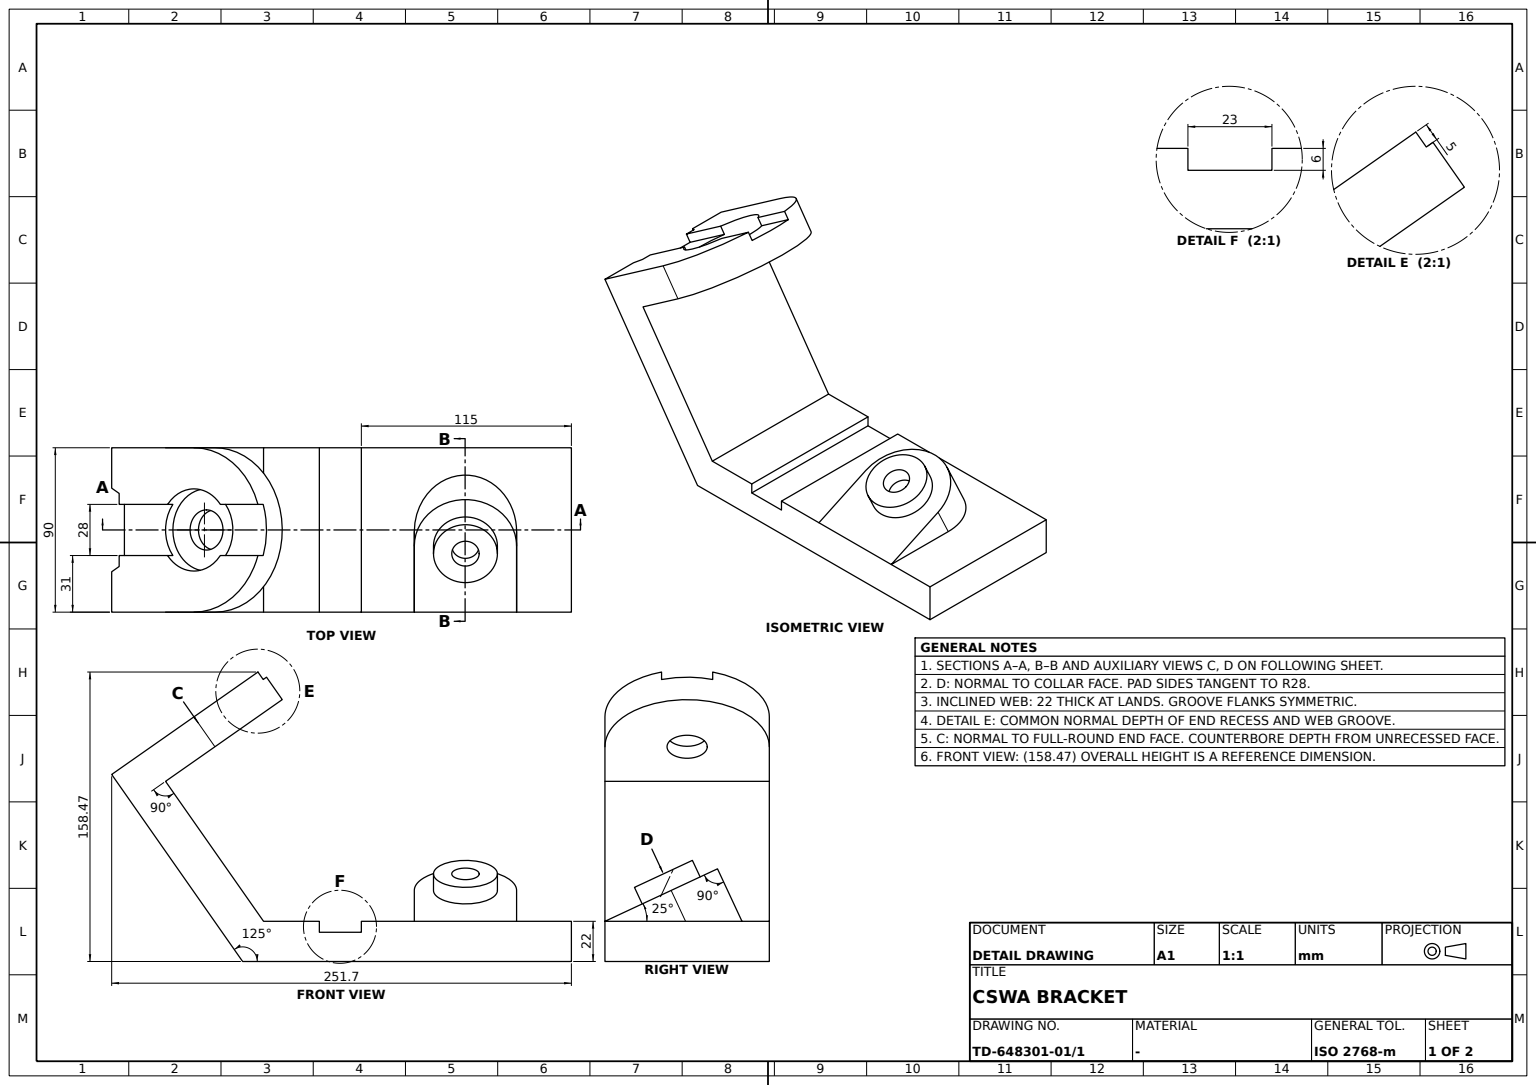
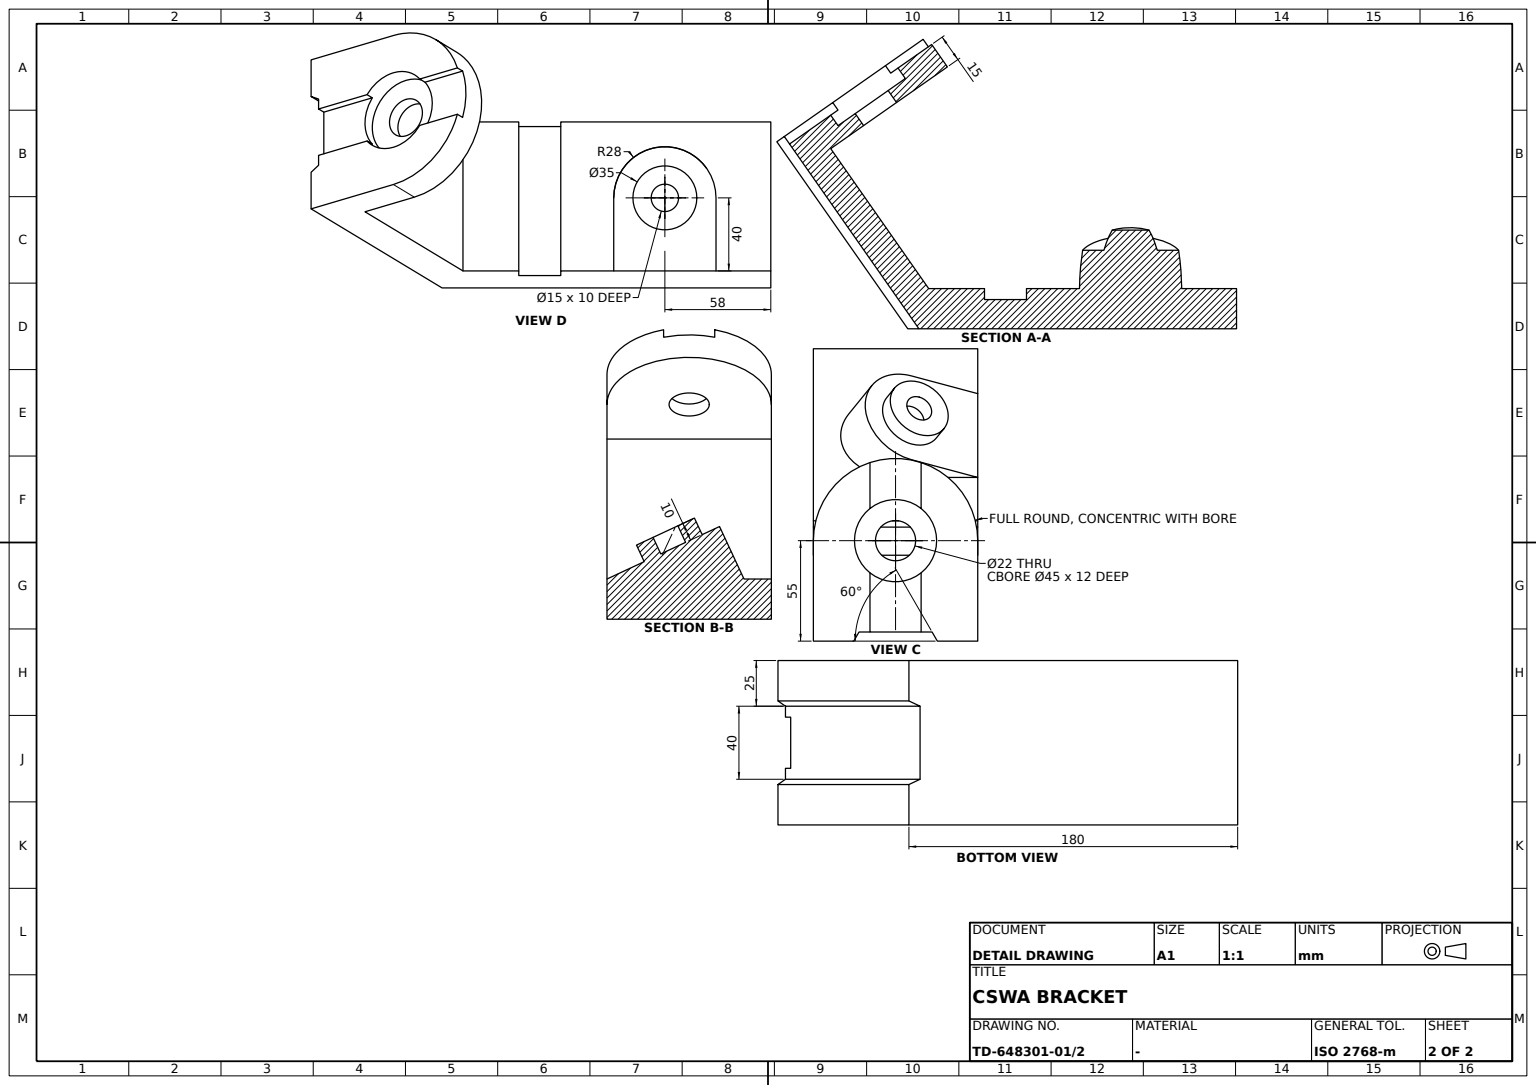
CATIA V5 part; units mm, degrees
ref_plane "Plane1" through (16.4638, 0, 35.3067) normal (-0.4226, 0, -0.9063) x (0, -1, 0)
sketch "Sketch1" plane through (0, 0, 0) normal (1, 0, 0) x (0, 1, 0)
  line L0 (0, 0) -> (180, 0)
  line L1 (180, 0) -> (180, 22)
  point P0 (180, 22)
  line L2 (0, 0) -> (-71.6971, 102.394)
  line L3 (-71.6971, 102.394) -> (-26.6437, 133.9407)
  line L4 (-26.6437, 133.9407) -> (-15.1722, 117.5577)
  point P1 (-15.1722, 117.5577)
  line L5 (-15.1722, 117.5577) -> (-42.2042, 98.6296)
  point P2 (-15.1722, 117.5577)
  point P3 (-42.2042, 98.6296)
  line L6 (-42.2042, 98.6296) -> (11.4525, 22)
  line L7 (11.4525, 22) -> (42, 22)
  point P4 (42, 22)
  line L8 (42, 22) -> (42, 16)
  line L9 (42, 16) -> (65, 16)
  line L10 (65, 16) -> (65, 22)
  point P5 (65, 22)
  line L11 (65, 22) -> (180, 22)
  dimension "length L0" = 180
  dimension "length L2" = 125
  dimension "angle L2 L0" = 55
  dimension "length L3" = 55
  dimension "length L4" = 20
  dimension "distance P3 L2" = 22
  dimension "distance P4 P0" = 138
  dimension "distance L7 L0" = 22
  dimension "length L8" = 6
  dimension "length L9" = 23
  constraint horizontal L0 x-axis
  constraint horizontal L7 x-axis
  constraint horizontal L9 x-axis
  constraint horizontal L11 x-axis
  constraint vertical L1 y-axis
  constraint vertical L8 y-axis
  constraint vertical L10 y-axis
  constraint perpendicularity L3 L2
  constraint parallelism L4 L2
  constraint parallelism L5 L3
  constraint parallelism L6 L2
  constraint coincidence P2 L4
  constraint coincidence P2 P1
  constraint coincidence P5 L7
extrude "Pad1" add sketch "Sketch1" along normal mid plane 90
sketch "Sketch2" plane through (16.4638, 0, 35.3067) normal (-0.4226, 0, -0.9063) x (0, -1, 0)
  line L0 (-150, -31.4862) -> (-150, 8.5138)
  point P0 (-150, -31.4862)
  line L1 (-180, -31.4862) -> (-65, -31.4862) construction
  line L2 (-180, 50.0815) -> (-180, -31.4862) construction
  line L3 (-94, 8.5138) -> (-94, -31.4862)
  arc A0 (-94, 8.5138) -> (-150, 8.5138) centre (-122, 8.5138) ccw
  line L4 (-94, -31.4862) -> (-150, -31.4862)
  dimension "length L0" = 40
  dimension "distance L0 L2" = 30
  dimension "radius A0" = 28
  constraint vertical L0 y-axis
  constraint vertical L3 y-axis
  constraint coincidence P0 L1
  constraint tangency A0 L0
  constraint horizontal L4 x-axis
extrude "Pad2" add sketch "Sketch2" along normal up to surface surface through (-45, 65, 22) normal (0, 0, 1)
sketch "Sketch3" plane through (16.4638, 0, 35.3067) normal (0.4226, 0, 0.9063) x (0, 1, 0)
  circle A0 centre (122, 8.5138) radius 17.5
  arc A1 (150, 8.5138) -> (94, 8.5138) centre (122, 8.5138) ccw construction
  dimension "radius A0" = 17.5
  constraint concentricity A0 A1
extrude "Pad3" add sketch "Sketch3" along normal blind 10
sketch "Sketch4" plane through (20.69, 0, 44.3698) normal (0.4226, 0, 0.9063) x (0, 1, 0)
  circle A0 centre (122, 8.5138) radius 7.5
  circle A1 centre (122, 8.5138) radius 17.5 construction
  dimension "radius A0" = 7.5
  constraint concentricity A0 A1
extrude "Pocket1" cut sketch "Sketch4" against normal blind 10
sketch "Sketch5" plane through (0, -71.6971, 102.394) normal (0, -0.5736, 0.8192) x (1, 0, 0)
  line L0 (-45, 55) -> (45, 55)
  arc A0 (-45, 55) -> (45, 55) centre (0, 55) cw
  point P0 (0, 55)
  dimension "distance P0 x axis" = 55
  dimension "radius A0" = 45
extrude "Pad4" add sketch "Sketch5" against normal blind 20
sketch "Sketch6" plane through (10.7099, -32.8491, 129.5956) normal (0, -0.5736, 0.8192) x (1, 0, 0)
  point P0 (-10.7099, 7.5754)
  arc A0 (34.2901, 7.5754) -> (-55.7099, 7.5754) centre (-10.7099, 7.5754) ccw construction
  constraint concentricity P0 A0
hole "Hole1" at (0, -26.6437, 133.9407) direction (0, 0.5736, -0.8192) diameter 22 depth 20 tip angle 120 counterbore diameter 45 counterbore depth 12
sketch "Sketch7" plane through (0, -71.6971, 102.394) normal (0, -0.5736, 0.8192) x (1, 0, 0)
  point P0 (0, 34.2056)
  line L0 (14, 107.6997) -> (14, -39.2885)
  line L1 (14, -39.2885) -> (-14, -39.2885)
  line L2 (-14, -39.2885) -> (-14, 107.6997)
  line L3 (-14, 107.6997) -> (14, 107.6997)
  dimension "length L1" = 28
  constraint coincidence P0 y-axis
  constraint vertical L0 y-axis
  constraint vertical L2 y-axis
  constraint horizontal L1 x-axis
  constraint horizontal L3 x-axis
  constraint equidistance L0 L2 P0
  constraint equidistance L1 L3 P0
extrude "Pocket2" cut sketch "Sketch7" against normal blind 5
sketch "Sketch8" plane through (0, -71.6971, 102.394) normal (0, -0.5736, 0.8192) x (1, 0, 0)
  line L0 (-20, 5) -> (20, 5)
  point P0 (0, 5)
  point P1 (-20, 5)
  point P2 (20, 5)
  line L1 (-20, 5) -> (-22.8868, 0)
  point P3 (-22.8868, 0)
  line L2 (-14, 72.6139) -> (-14, 97.7668) construction
  line L3 (-45, 0) -> (45, 0) construction
  point P4 (22.8868, 0)
  point P5 (20, 5)
  line L4 (20, 5) -> (22.8868, 0)
  line L5 (-22.8868, 0) -> (22.8868, 0)
  dimension "length L0" = 40
  dimension "distance L0 x axis" = 5
  dimension "angle L1 L2" = 30
  constraint midpoint L0 P0
  constraint coincidence P0 y-axis
  constraint coincidence P3 L3
  constraint coincidence P2 P5
  constraint horizontal L0 x-axis
  constraint horizontal L5 x-axis
  constraint symmetry P3 P4 y-axis
  constraint symmetry P1 P5 y-axis
  constraint symmetry L1 L4 y-axis
extrude "Pocket3" cut sketch "Sketch8" against normal through all
